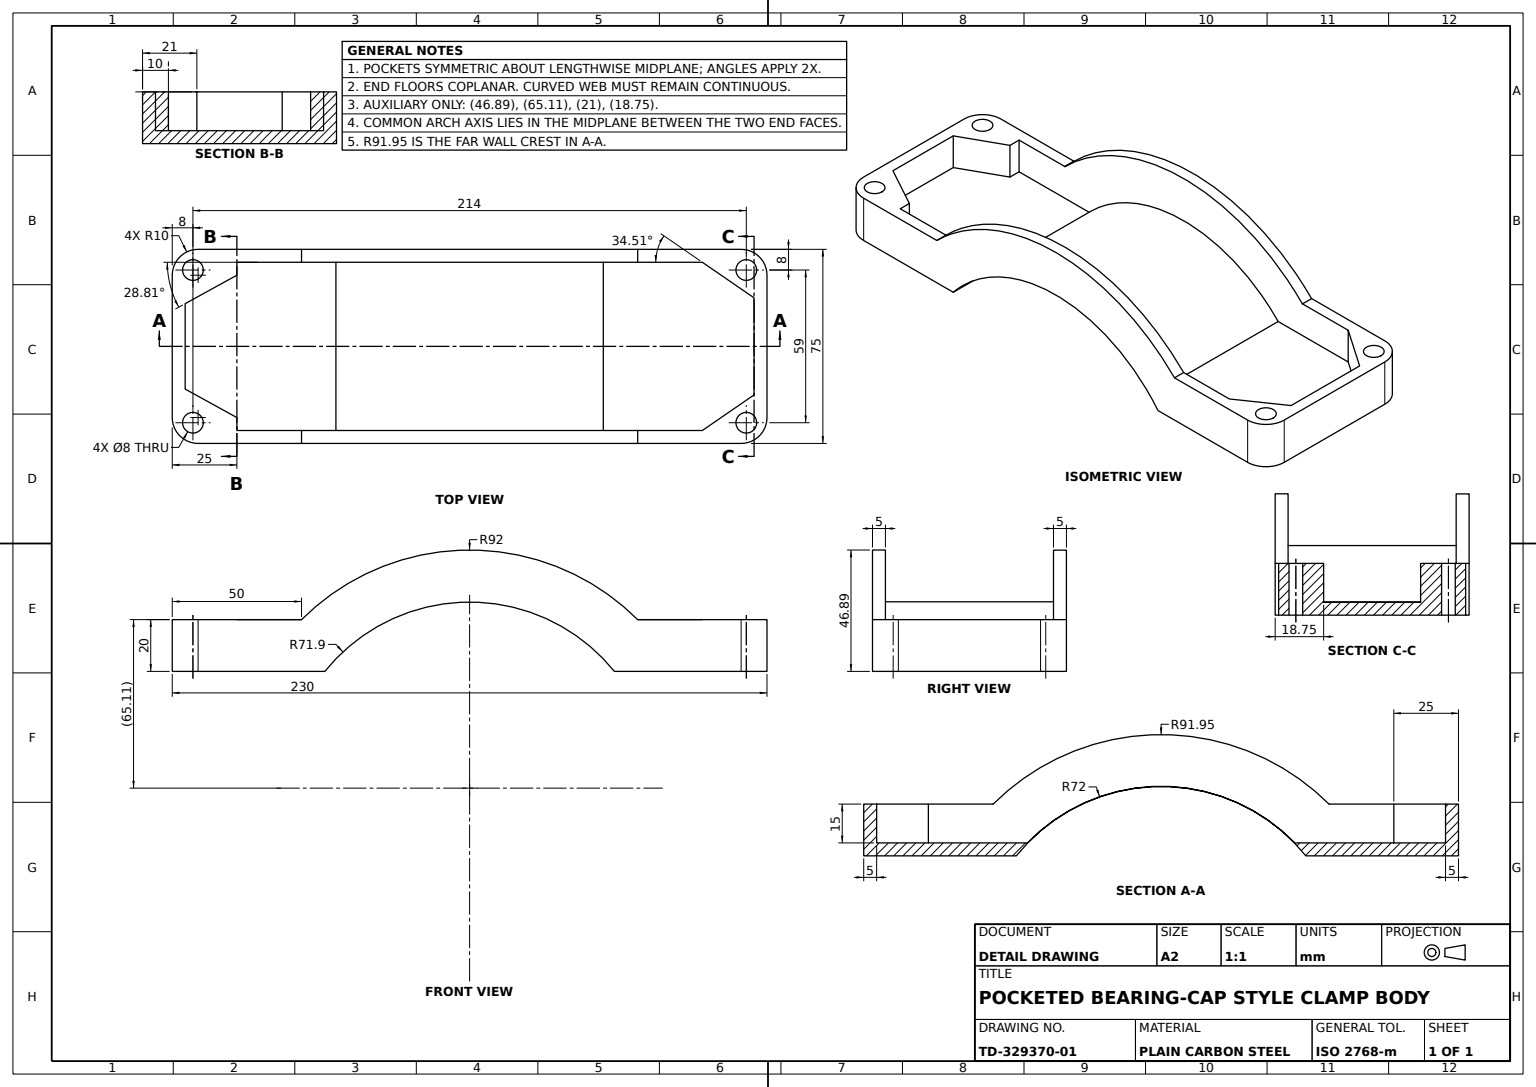
from build123d import *

# Parameters (mm, degrees)
SIDE_WALL_DEPTH           = 5
END_FLANGE_A_DEPTH        = 50
FLANGE_A_POCKET_DEPTH     = 15
ARCH_SHELL_DEPTH          = 75
SIDE_START                = -5
SIDE_WALL_EXTENSION_DEPTH = 5
FLANGE_START              = -75
FLANGE_A_RIM_DEPTH        = 75
END_FLANGE_B_SKETCH_W     = 75
END_FLANGE_B_SKETCH_H     = 20
END_FLANGE_B_DEPTH        = 50
FLANGE_B_POCKET_DEPTH     = 15
FLANGE_B_RIM_DEPTH        = 75
BOLT_HOLES_SKETCH_R       = 4
BOLT_HOLES_4X_DEPTH       = 75
CORNER_FILLETS_R10_A_R    = 10
CORNER_FILLETS_R10_B_R    = 10
CORNER_FILLETS_R10_C_R    = 10
CORNER_FILLETS_R10_D_R    = 10


with BuildPart() as part:
    # Side Wall Profile Sketch → Side Wall (new body)
    with BuildSketch(Plane(origin=(0, 0, 0), x_dir=(0, 0, -1), z_dir=(1, 0, 0))):
        with BuildLine():
            ThreePointArc((56.118661154, 45.107603243), (0, 72), (-56.118661154, 45.107603243))
            Line((-56.118661154, 45.107603243), (-115, 45.107603243))
            Line((-115, 45.107603243), (-115, 65.107603243))
            Line((-115, 65.107603243), (-65, 65.107603243))
            ThreePointArc((-65, 65.107603243), (0, 92), (65, 65.107603243))
            Line((65, 65.107603243), (115, 65.107603243))
            Line((115, 65.107603243), (115, 45.107603243))
            Line((115, 45.107603243), (95, 45.107603243))
            Line((95, 45.107603243), (56.118661154, 45.107603243))
        make_face()
    extrude(amount=-SIDE_WALL_DEPTH)

    # End Flange A Sketch → End Flange A (add)
    with BuildSketch(Plane.XY.offset(115)):
        Polygon((0, 45.107603243), (-75, 45.107603243), (-75, 65.107603243), (-5, 65.107603243), (0, 65.107603243), align=None)
    extrude(amount=-END_FLANGE_A_DEPTH)

    # Flange A Pocket Sketch → Flange A Pocket (cut)
    with BuildSketch(Plane(origin=(0, 65.107603243, 0), x_dir=(1, 0, 0), z_dir=(0, 1, 0))):
        Polygon((-10, -90), (-5, -90), (-5, -65), (-70, -65), (-70, -90), (-65, -90), (-54, -110), (-21, -110), align=None)
    extrude(amount=-FLANGE_A_POCKET_DEPTH, mode=Mode.SUBTRACT)

    # Arch Shell Sketch → Arch Shell (add)
    with BuildSketch(Plane(origin=(0, 0, 0), x_dir=(0, 0, -1), z_dir=(1, 0, 0))):
        with BuildLine():
            Line((-56.118661154, 45.107603243), (-55.986211495, 45.107603243))
            ThreePointArc((-55.986211495, 45.107603243), (0, 71.896813197), (55.986211495, 45.107603243))
            Line((55.986211495, 45.107603243), (56.118661154, 45.107603243))
            ThreePointArc((56.118661154, 45.107603243), (0, 72), (-56.118661154, 45.107603243))
        make_face()
    extrude(amount=-ARCH_SHELL_DEPTH)

    # Side Wall Extension Sketch → Side Wall Extension (add)
    with BuildSketch(Plane.ZY.offset(75).offset(SIDE_START)):
        with BuildLine():
            ThreePointArc((-65, 65.043834782), (-73.247030889, 55.592921393), (-80.131171043, 45.107603243))
            Line((-80.131171043, 45.107603243), (-65, 45.107603243))
            Line((-65, 45.107603243), (-56.118661154, 45.107603243))
            ThreePointArc((-56.118661154, 45.107603243), (0, 72), (56.118661154, 45.107603243))
            Line((56.118661154, 45.107603243), (65, 45.107603243))
            Line((65, 45.107603243), (65, 65.043834782))
            ThreePointArc((65, 65.043834782), (0, 91.95488265), (-65, 65.043834782))
        make_face()
    extrude(amount=SIDE_WALL_EXTENSION_DEPTH)

    # Flange A Rim Sketch → Flange A Rim (add)
    with BuildSketch(Plane.ZY.offset(75).offset(FLANGE_START)):
        with BuildLine():
            Line((55.986211495, 45.107603243), (65, 45.107603243))
            Line((65, 45.107603243), (65, 50.107603243))
            Line((65, 50.107603243), (51.559478713, 50.107603243))
            ThreePointArc((51.559478713, 50.107603243), (53.830928569, 47.659027238), (55.986211495, 45.107603243))
        make_face()
    extrude(amount=FLANGE_A_RIM_DEPTH)

    # End Flange B Sketch → End Flange B (add)
    with BuildSketch(Plane(origin=(0, 0, -115), x_dir=(-1, 0, 0), z_dir=(0, 0, -1))):
        with Locations((37.5, 55.107603243)):
            Rectangle(END_FLANGE_B_SKETCH_W, END_FLANGE_B_SKETCH_H)
    extrude(amount=-END_FLANGE_B_DEPTH)

    # Flange B Pocket Sketch → Flange B Pocket (cut)
    with BuildSketch(Plane(origin=(0, 65.107603243, 0), x_dir=(1, 0, 0), z_dir=(0, 1, 0))):
        Polygon((-56.25, 110), (-70, 90), (-70, 65), (-5, 65), (-5, 90), (-18.75, 110), (-37.5, 110), align=None)
    extrude(amount=-FLANGE_B_POCKET_DEPTH, mode=Mode.SUBTRACT)

    # Flange B Rim Sketch → Flange B Rim (add)
    with BuildSketch(Plane(origin=(0, 0, 0), x_dir=(0, 0, -1), z_dir=(1, 0, 0))):
        with BuildLine():
            Line((65, 45.107603243), (65, 50.107603243))
            Line((65, 50.107603243), (51.559478713, 50.107603243))
            ThreePointArc((51.559478713, 50.107603243), (53.830928569, 47.659027238), (55.986211495, 45.107603243))
            Line((55.986211495, 45.107603243), (65, 45.107603243))
        make_face()
    extrude(amount=-FLANGE_B_RIM_DEPTH)

    # Bolt Holes Sketch → Bolt Holes 4x (cut)
    with BuildSketch(Plane(origin=(0, 65.107603243, 0), x_dir=(1, 0, 0), z_dir=(0, 1, 0))):
        with Locations(Location((-8, 107, 0), (0, 0, 270))):
            Circle(BOLT_HOLES_SKETCH_R)
        with Locations(Location((-67, 107, 0), (0, 0, 270))):
            Circle(BOLT_HOLES_SKETCH_R)
        with Locations(Location((-8, -107, 0), (0, 0, 270))):
            Circle(BOLT_HOLES_SKETCH_R)
        with Locations(Location((-67, -107, 0), (0, 0, 270))):
            Circle(BOLT_HOLES_SKETCH_R)
    extrude(amount=-BOLT_HOLES_4X_DEPTH, mode=Mode.SUBTRACT)

    # Corner Fillets R10 A
    corner_fillets_r10_a_edges = [part.edges().sort_by_distance(p)[0] for p in [
        (0, 55.107603243, 115),
    ]]
    fillet(corner_fillets_r10_a_edges, radius=CORNER_FILLETS_R10_A_R)

    # Corner Fillets R10 B
    corner_fillets_r10_b_edges = [part.edges().sort_by_distance(p)[0] for p in [
        (-75, 55.107603243, 115),
    ]]
    fillet(corner_fillets_r10_b_edges, radius=CORNER_FILLETS_R10_B_R)

    # Corner Fillets R10 C
    corner_fillets_r10_c_edges = [part.edges().sort_by_distance(p)[0] for p in [
        (-75, 55.107603243, -115),
    ]]
    fillet(corner_fillets_r10_c_edges, radius=CORNER_FILLETS_R10_C_R)

    # Corner Fillets R10 D
    corner_fillets_r10_d_edges = [part.edges().sort_by_distance(p)[0] for p in [
        (0, 55.107603243, -115),
    ]]
    fillet(corner_fillets_r10_d_edges, radius=CORNER_FILLETS_R10_D_R)


solid = part.part
